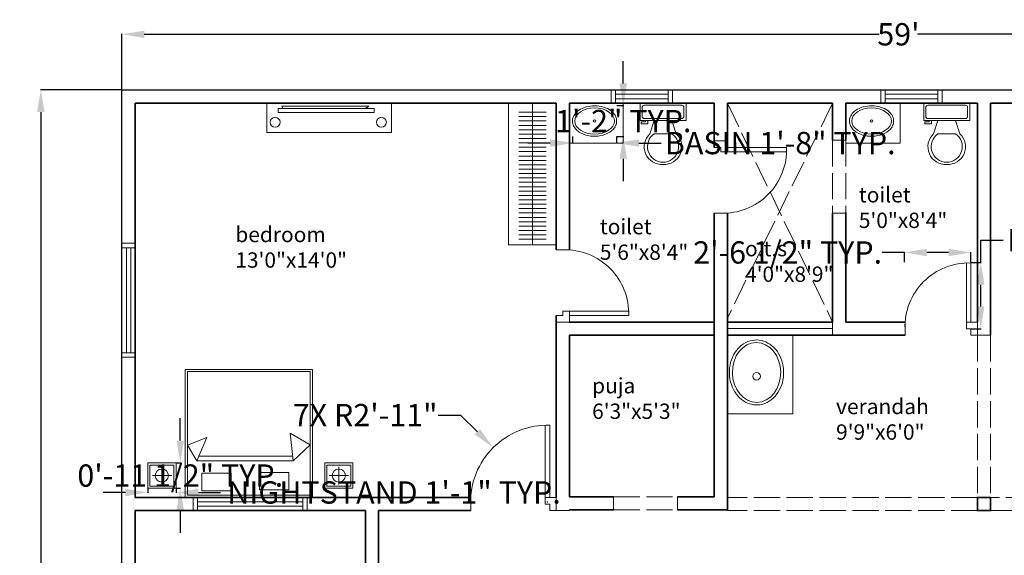
# Model space of a CAD drawing. Units: inches. Extents: x 29 to 4581, y 6 to 2196.
# Tile 2 of 3: x 3825 to 4274, y 1948 to 2192. Entities that reach past the tile are written whole.
import ezdxf

# ---------------------------------------------------------------- set-up
doc = ezdxf.new("R2010")
doc.units = ezdxf.units.IN
doc.header["$MEASUREMENT"] = 0
doc.linetypes.add('ACAD_ISO02W100', pattern=[15, 12, -3])
for name, color, linetype, lineweight in [('A-ANNO-DIMS', 2, 'Continuous', 18), ('A-DOOR', 3, 'Continuous', 18), ('A-EQPM', 9, 'Continuous', 18), ('A-FLOR-CASE', 8, 'Continuous', 18), ('A-FLOR-CASE-PATT', 8, 'Continuous', 13), ('A-FLOR-FIXT', 9, 'Continuous', 18), ('A-FLOR-OPEN', 8, 'ACAD_ISO02W100', 13), ('A-GLAZ', 4, 'Continuous', 18), ('A-WALL', 7, 'Continuous', 35), ('A-WALL-OVHD', 8, 'ACAD_ISO02W100', 18), ('C-PROP', 8, 'Continuous', 25)]:
    doc.layers.add(name, color=color, linetype=linetype, lineweight=lineweight)
for name, color, linetype, lineweight, true_color in [('A-AREA-IDEN', 41, 'Continuous', 18, 0xf4ee51), ('A-COLS', 240, 'Continuous', 35, 0xed1f24), ('A-FURN', 31, 'Continuous', 18, 0xfecc66)]:
    doc.layers.add(name, color=color, linetype=linetype, lineweight=lineweight, true_color=true_color)
doc.styles.get("Standard").update_dxf_attribs({"font": 'arial.ttf'})
doc.dimstyles.get("Standard").update_dxf_attribs({"dimtxt": 10.18, "dimasz": 10.18, "dimexe": 0.18, "dimexo": 0.0625, "dimgap": 0.09, "dimtad": 0, "dimtih": 1, "dimtoh": 1, "dimdec": 0, "dimzin": 0, "dimdsep": 46, "dimlunit": 3, "dimtxsty": 'Standard', "dimcen": 0.09, "dimadec": 0, "dimazin": 0, "dimtfac": 1, "dimtdec": 0, "dimtofl": 0, "dimtmove": 0, "dimatfit": 3, "dimfxl": 1, "dimtolj": 1, "dimtzin": 0, "dimarcsym": 0})

# ---------------------------------------------------------------- blocks, each defined once
blk = doc.blocks.new('*U2')
for p, q in [((9.5, -6), (9.5, -2)), ((-10, -8.5), (-8, -8.5)), ((-10, -9.5), (-10, -8.5)), ((-8, -8.5), (-8, -8)), ((-7, -8), (-7, -9.5)), ((-4, -8), (-6, -14)), ((4, -8), (6, -14)), ((-7, -9.5), (-10, -9.5)), ((4, -14), (-4, -14))]:
    blk.add_line(p, q)
blk.add_lwpolyline([(10.5, -8), (10.5, 0), (-10.5, 0), (-10.5, -8)], close=True)
for points in [[(-9.5, -2), (-9.5, -6)], [(8.5, -1), (-8.5, -1)], [(-8.5, -7), (8.5, -7)]]:
    blk.add_lwpolyline(points)
for centre, radius, start, end in [((-8.625, -1.875), 0.8839, 81.8699, 188.1301), ((8.625, -1.875), 0.8839, 351.8699, 98.1301), ((-8.625, -6.125), 0.8839, 171.869898, 278.1301), ((8.625, -6.125), 0.8839, 261.8699, 8.1301), ((-0.4772, -19.9188), 8.0953, 133.01722, 273.38), ((0.0374, -19.8731), 7.127, 124.50543, 269.7), ((-0.0373, -19.8731), 7.127, 270.3, 55.4946), ((0.4773, -19.9188), 8.0953, 266.62, 46.9828)]:
    blk.add_arc(centre, radius, start, end)
blk = doc.blocks.new('*D7')
at = {"layer": 'A-ANNO-DIMS', "color": 0, "lineweight": -2, "transparency": 16777216}
for p, q in [((3871.98, 2160.26), (3871.98, 2185.77)), ((3882.16, 2185.59), (4217.25, 2185.59)), ((4569.8, 2185.59), (4234.7, 2185.59)), ((4579.98, 2160.26), (4579.98, 2185.77))]:
    blk.add_line(p, q, dxfattribs=at)
at = {"layer": 'A-ANNO-DIMS', "color": 0, "transparency": 16777216}
for points in [[(3882.16, 2187.28), (3882.16, 2183.89), (3871.98, 2185.59)], [(4569.8, 2187.28), (4569.8, 2183.89), (4579.98, 2185.59)]]:
    blk.add_solid(points, dxfattribs=at)
at = {"layer": 'Defpoints', "color": 0, "transparency": 16777216}
for p in [(4579.98, 2185.59), (3871.98, 2160.2), (4579.98, 2160.2)]:
    blk.add_point(p, dxfattribs=at)
at = {"layer": 'A-ANNO-DIMS', "color": 0, "transparency": 16777216, "insert": (4225.98, 2185.59), "char_height": 10.18, "attachment_point": 5}
blk.add_mtext("\\A1;59'", dxfattribs=at)
blk = doc.blocks.new('*D8')
at = {"layer": 'A-ANNO-DIMS', "color": 0, "lineweight": -2, "transparency": 16777216}
for p, q in [((3871.91, 2160.26), (3834.8, 2160.26)), ((3834.98, 2150.08), (3834.98, 1865.52)), ((3834.98, 1570.38), (3834.98, 1854.94)), ((3871.91, 1560.2), (3834.8, 1560.2))]:
    blk.add_line(p, q, dxfattribs=at)
at = {"layer": 'A-ANNO-DIMS', "color": 0, "transparency": 16777216}
for points in [[(3833.29, 2150.08), (3836.68, 2150.08), (3834.98, 2160.26)], [(3833.29, 1570.38), (3836.68, 1570.38), (3834.98, 1560.2)]]:
    blk.add_solid(points, dxfattribs=at)
at = {"layer": 'Defpoints', "color": 0, "transparency": 16777216}
for p in [(3834.98, 2160.26), (3871.98, 2160.26), (3871.98, 1560.2)]:
    blk.add_point(p, dxfattribs=at)
at = {"layer": 'A-ANNO-DIMS', "color": 0, "transparency": 16777216, "insert": (3834.98, 1860.23), "char_height": 10.18, "attachment_point": 5}
blk.add_mtext("\\A1;50'", dxfattribs=at)
blk = doc.blocks.new('DOOR-36IN')
for p, q in [((34.01, 0), (34.01, 36)), ((36.01, 3), (36.01, 36)), ((34.01, 0), (36.01, 0))]:
    blk.add_line(p, q)
blk.add_arc((35.01, 1), 35.01, 88.3634, 181.6366)
blk = doc.blocks.new('DOOR-30IN')
for p, q in [((0, 2), (30, 2)), ((0, 2), (0, 0)), ((3, 0), (30, 0))]:
    blk.add_line(p, q)
blk.add_arc((1, 1), 29.02, 358.0251, 91.9749)
blk = doc.blocks.new('WIN-48')
for p, q in [((0, 6), (0, 0)), ((2, 6), (2, 0)), ((50, 6), (50, 0)), ((52, 6), (52, 0)), ((2, 4), (50, 4)), ((2, 2), (50, 2))]:
    blk.add_line(p, q)
blk = doc.blocks.new('WIN-24')
for p, q in [((6, 28), (0, 28)), ((6, 26), (0, 26)), ((2, 26), (2, 2)), ((4, 26), (4, 2)), ((6, 2), (0, 2)), ((6, 0), (0, 0))]:
    blk.add_line(p, q)
blk = doc.blocks.new('BASIN-OVAL')
blk.add_circle((10.07, 6.96), 0.572)
blk.add_ellipse((10.07, 6.96), major_axis=(9.07, 0), ratio=0.657752)
blk.add_open_spline([(20.13, 6.96), (20.13, 7.48), (20.05, 7.99), (19.74, 8.98), (19.5, 9.46), (18.6, 10.81), (17.74, 11.59), (15.67, 12.84), (14.47, 13.31), (11.89, 13.88), (10.52, 13.98), (7.83, 13.82), (6.51, 13.55), (4.11, 12.67), (3.03, 12.06), (1.49, 10.71), (0.93, 10.02), (0.24, 8.64), (0.05, 7.96), (-0.03, 6.59), (0.07, 5.9), (0.54, 4.6), (0.91, 3.98), (1.85, 2.86), (2.43, 2.36), (4.23, 1.16), (5.63, 0.61), (8.62, -0.01), (10.22, -0.08), (13.3, 0.28), (14.78, 0.7), (17.33, 1.99), (18.39, 2.86), (19.54, 4.5), (19.85, 5.16), (20.09, 6.22), (20.13, 6.59), (20.13, 6.96)], degree=3, knots=[0, 0, 0, 0, 0.206246, 0.206246, 0.412492, 0.412492, 0.829146, 0.829146, 1.245799, 1.245799, 1.662453, 1.662453, 2.079106, 2.079106, 2.495759, 2.495759, 2.824502, 2.824502, 3.099346, 3.099346, 3.37419, 3.37419, 3.649034, 3.649034, 3.923877, 3.923877, 4.405635, 4.405635, 4.887392, 4.887392, 5.369149, 5.369149, 5.850906, 5.850906, 6.134068, 6.134068, 6.283185, 6.283185, 6.283185, 6.283185])
blk = doc.blocks.new('NIGHTSTAND-WIDE')
for p, q in [((6.43, 9.73), (6.43, 1.64)), ((2.09, 5.78), (10.92, 5.78))]:
    blk.add_line(p, q)
for points in [[(0, 11.56), (12.87, 11.56), (12.87, 0), (0, 0)], [(1, 10.56), (11.87, 10.56), (11.87, 1), (1, 1)]]:
    blk.add_lwpolyline(points, close=True)
blk.add_circle((6.43, 5.78), 2.99)
blk = doc.blocks.new('*D28')
at = {"layer": 'A-ANNO-DIMS', "color": 0, "lineweight": -2, "transparency": 16777216}
for p, q in [((4263.52, 2081.47), (4263.52, 2091.65)), ((4263.52, 2091.65), (4273.7, 2091.65)), ((4259.04, 2081.47), (4263.7, 2081.47)), ((4263.52, 2061.38), (4263.52, 2071.29)), ((4259.04, 2051.2), (4263.7, 2051.2))]:
    blk.add_line(p, q, dxfattribs=at)
at = {"layer": 'A-ANNO-DIMS', "color": 0, "transparency": 16777216}
for points in [[(4261.82, 2071.29), (4265.21, 2071.29), (4263.52, 2081.47)], [(4261.82, 2061.38), (4265.21, 2061.38), (4263.52, 2051.2)]]:
    blk.add_solid(points, dxfattribs=at)
at = {"layer": 'Defpoints', "color": 0, "transparency": 16777216}
for p in [(4258.98, 2081.47), (4263.52, 2081.47), (4258.98, 2051.2)]:
    blk.add_point(p, dxfattribs=at)
at = {"layer": 'A-ANNO-DIMS', "color": 0, "transparency": 16777216, "insert": (4339.73, 2091.65), "char_height": 10.18, "attachment_point": 5}
blk.add_mtext('\\A1;DOOR 2\'-6 1/2" TYP.', dxfattribs=at)
blk = doc.blocks.new('*D29')
at = {"layer": 'A-ANNO-DIMS', "color": 0, "lineweight": -2, "transparency": 16777216}
for p, q in [((4228.7, 2086.02), (4218.52, 2086.02)), ((4228.7, 2081.54), (4228.7, 2086.2)), ((4248.8, 2086.02), (4238.88, 2086.02)), ((4258.98, 2081.54), (4258.98, 2086.2))]:
    blk.add_line(p, q, dxfattribs=at)
at = {"layer": 'A-ANNO-DIMS', "color": 0, "transparency": 16777216}
for points in [[(4238.88, 2087.71), (4238.88, 2084.32), (4228.7, 2086.02)], [(4248.8, 2087.71), (4248.8, 2084.32), (4258.98, 2086.02)]]:
    blk.add_solid(points, dxfattribs=at)
at = {"layer": 'Defpoints', "color": 0, "transparency": 16777216}
for p in [(4228.7, 2086.02), (4228.7, 2081.47), (4258.98, 2081.47)]:
    blk.add_point(p, dxfattribs=at)
at = {"layer": 'A-ANNO-DIMS', "color": 0, "transparency": 16777216, "insert": (4175.46, 2086.02), "char_height": 10.18, "attachment_point": 5}
blk.add_mtext('\\A1;2\'-6 1/2" TYP.', dxfattribs=at)
blk = doc.blocks.new('*D34')
at = {"layer": 'A-ANNO-DIMS', "color": 0, "lineweight": -2, "transparency": 16777216}
for p, q in [((4077.33, 2138.9), (4077.33, 2135.76)), ((4097.5, 2138.9), (4097.5, 2135.76)), ((4067.15, 2135.94), (4056.97, 2135.94)), ((4107.68, 2135.94), (4117.86, 2135.94))]:
    blk.add_line(p, q, dxfattribs=at)
at = {"layer": 'A-ANNO-DIMS', "color": 0, "transparency": 16777216}
for points in [[(4067.15, 2137.64), (4067.15, 2134.24), (4077.33, 2135.94)], [(4107.68, 2137.64), (4107.68, 2134.24), (4097.5, 2135.94)]]:
    blk.add_solid(points, dxfattribs=at)
at = {"layer": 'Defpoints', "color": 0, "transparency": 16777216}
for p in [(4077.33, 2138.97), (4097.5, 2138.97), (4097.5, 2135.94)]:
    blk.add_point(p, dxfattribs=at)
at = {"layer": 'A-ANNO-DIMS', "color": 0, "transparency": 16777216, "insert": (4172.07, 2135.94), "char_height": 10.18, "attachment_point": 5}
blk.add_mtext('\\A1;BASIN 1\'-8" TYP.', dxfattribs=at)
blk = doc.blocks.new('*D35')
at = {"layer": 'A-ANNO-DIMS', "color": 0, "lineweight": -2, "transparency": 16777216}
for p, q in [((4100.53, 2163.21), (4100.53, 2173.39)), ((4097.56, 2153.03), (4100.71, 2153.03)), ((4097.56, 2138.97), (4100.71, 2138.97)), ((4100.53, 2128.79), (4100.53, 2118.61))]:
    blk.add_line(p, q, dxfattribs=at)
at = {"layer": 'A-ANNO-DIMS', "color": 0, "transparency": 16777216}
for points in [[(4098.83, 2163.21), (4102.22, 2163.21), (4100.53, 2153.03)], [(4098.83, 2128.79), (4102.22, 2128.79), (4100.53, 2138.97)]]:
    blk.add_solid(points, dxfattribs=at)
at = {"layer": 'Defpoints', "color": 0, "transparency": 16777216}
for p in [(4097.5, 2153.03), (4100.53, 2153.03), (4097.5, 2138.97)]:
    blk.add_point(p, dxfattribs=at)
at = {"layer": 'A-ANNO-DIMS', "color": 0, "transparency": 16777216, "insert": (4100.53, 2146), "char_height": 10.18, "attachment_point": 5}
blk.add_mtext('\\A1;1\'-2" TYP.', dxfattribs=at)
blk = doc.blocks.new('*D40')
at = {"layer": 'A-ANNO-DIMS', "color": 0, "lineweight": -2, "transparency": 16777216}
for p, q in [((3873.56, 1976.48), (3863.38, 1976.48)), ((3883.74, 1978.35), (3883.74, 1976.3)), ((3896.61, 1978.35), (3896.61, 1976.3)), ((3906.79, 1976.48), (3916.97, 1976.48))]:
    blk.add_line(p, q, dxfattribs=at)
at = {"layer": 'A-ANNO-DIMS', "color": 0, "transparency": 16777216}
for points in [[(3873.56, 1978.17), (3873.56, 1974.78), (3883.74, 1976.48)], [(3906.79, 1978.17), (3906.79, 1974.78), (3896.61, 1976.48)]]:
    blk.add_solid(points, dxfattribs=at)
at = {"layer": 'Defpoints', "color": 0, "transparency": 16777216}
for p in [(3883.74, 1978.41), (3896.61, 1978.41), (3896.61, 1976.48)]:
    blk.add_point(p, dxfattribs=at)
at = {"layer": 'A-ANNO-DIMS', "color": 0, "transparency": 16777216, "insert": (3996.03, 1976.48), "char_height": 10.18, "attachment_point": 5}
blk.add_mtext('\\A1;NIGHTSTAND 1\'-1" TYP.', dxfattribs=at)
blk = doc.blocks.new('*D41')
at = {"layer": 'A-ANNO-DIMS', "color": 0, "lineweight": -2, "transparency": 16777216}
for p, q in [((3898.54, 2000.15), (3898.54, 2010.33)), ((3896.67, 1989.97), (3898.72, 1989.97)), ((3896.67, 1978.41), (3898.72, 1978.41)), ((3898.54, 1968.23), (3898.54, 1958.05))]:
    blk.add_line(p, q, dxfattribs=at)
at = {"layer": 'A-ANNO-DIMS', "color": 0, "transparency": 16777216}
for points in [[(3896.84, 2000.15), (3900.23, 2000.15), (3898.54, 1989.97)], [(3896.84, 1968.23), (3900.23, 1968.23), (3898.54, 1978.41)]]:
    blk.add_solid(points, dxfattribs=at)
at = {"layer": 'Defpoints', "color": 0, "transparency": 16777216}
for p in [(3896.61, 1989.97), (3898.54, 1989.97), (3896.61, 1978.41)]:
    blk.add_point(p, dxfattribs=at)
at = {"layer": 'A-ANNO-DIMS', "color": 0, "transparency": 16777216, "insert": (3898.54, 1984.19), "char_height": 10.18, "attachment_point": 5}
blk.add_mtext('\\A1;0\'-11 1/2" TYP.', dxfattribs=at)
blk = doc.blocks.new('*D48')
at = {"layer": 'A-ANNO-DIMS', "color": 0, "lineweight": -2, "transparency": 16777216}
for p, q in [((4016.18, 2011.81), (4026.36, 2011.81)), ((4026.36, 2011.81), (4034.02, 2004.15)), ((4065.89, 1972.2), (4066.07, 1972.2)), ((4065.98, 1972.11), (4065.98, 1972.29))]:
    blk.add_line(p, q, dxfattribs=at)
at = {"layer": 'A-ANNO-DIMS', "color": 0, "transparency": 16777216}
blk.add_solid([(4035.22, 2005.35), (4032.82, 2002.95), (4041.22, 1996.96)], dxfattribs=at)
at = {"layer": 'Defpoints', "color": 0, "transparency": 16777216}
for p in [(4041.22, 1996.96), (4065.98, 1972.2)]:
    blk.add_point(p, dxfattribs=at)
at = {"layer": 'A-ANNO-DIMS', "color": 0, "transparency": 16777216, "insert": (3982.84, 2011.81), "char_height": 10.18, "attachment_point": 5}
blk.add_mtext('\\A1;7X R2\'-11"', dxfattribs=at)

msp = doc.modelspace()

# ---------------------------------------------------------------- hatches: boundary and pattern name
at = {"layer": 'A-FLOR-CASE-PATT'}
h = msp.add_hatch(dxfattribs=at)
h.set_pattern_fill('ANSI31', color=256, scale=16.0003, angle=-45, style=0)
h.paths.add_polyline_path([(4052.97, 2091.04), (4065.4, 2091.04), (4065.4, 2151.04), (4052.97, 2151.04)])

# ---------------------------------------------------------------- linework, layer by layer
at = {"layer": 'A-COLS'}
msp.add_lwpolyline([(4267.98, 1974.2), (4261.98, 1974.2), (4261.98, 1968.2), (4267.98, 1968.2)], close=True, dxfattribs=at)
at = {"layer": 'A-DOOR'}
for p, q in [((4147.98, 2136.93), (4141.98, 2136.93)), ((4144.98, 2133.93), (4141.98, 2133.93)), ((4147.98, 2103.93), (4141.98, 2103.93)), ((4075.98, 2087.2), (4069.98, 2087.2)), ((4072.98, 2057.2), (4069.98, 2057.2)), ((4075.98, 2059.2), (4075.98, 2054.2)), ((4075.98, 2054.2), (4069.98, 2054.2)), ((4228.98, 2054.2), (4228.98, 2048.2)), ((4256.98, 2054.2), (4261.98, 2054.2)), ((4261.98, 2054.2), (4261.98, 2048.2)), ((4258.98, 2051.2), (4258.98, 2048.2)), ((4258.98, 2048.2), (4261.98, 2048.2)), ((4030.98, 1974.2), (4030.98, 1968.2)), ((4064.98, 1974.2), (4069.98, 1974.2)), ((4066.98, 1971.2), (4066.98, 1968.2)), ((4069.98, 1974.2), (4069.98, 1968.2)), ((4066.98, 1968.2), (4075.98, 1968.2))]:
    msp.add_line(p, q, dxfattribs=at)
at = {"layer": 'A-EQPM'}
for p, q in [((3945.29, 2151.69), (3944.84, 2152.73)), ((3944.84, 2152.73), (3984.49, 2152.73)), ((3984.49, 2152.73), (3982.98, 2151.69))]:
    msp.add_line(p, q, dxfattribs=at)
for points in [[(3938.02, 2154.2), (3994.84, 2154.2), (3994.84, 2140.8), (3938.02, 2140.8)], [(3943.21, 2151.69), (3987.01, 2151.69), (3987.01, 2149.92), (3943.21, 2149.92)]]:
    msp.add_lwpolyline(points, close=True, dxfattribs=at)
for centre in [(3941.79, 2145.45), (3990.24, 2145.45)]:
    msp.add_circle(centre, 2.26, dxfattribs=at)
at = {"layer": 'A-FLOR-CASE'}
msp.add_line((4059.09, 2154.2), (4059.09, 2089.54), dxfattribs=at)
msp.add_lwpolyline([(4069.98, 2154.2), (4048.2, 2154.2), (4048.2, 2089.54), (4069.98, 2089.54)], close=True, dxfattribs=at)
at = {"layer": 'A-FLOR-FIXT'}
for p, q in [((4100.43, 2154.2), (4100.43, 2135.9)), ((4226.71, 2154.2), (4226.71, 2135.9)), ((4100.43, 2135.9), (4075.98, 2135.9)), ((4226.71, 2135.9), (4202.26, 2135.9)), ((4177.83, 2048.2), (4177.83, 2012.33)), ((4177.83, 2012.33), (4147.98, 2012.33))]:
    msp.add_line(p, q, dxfattribs=at)
msp.add_circle((4161.28, 2029.53), 1.74, dxfattribs=at)
msp.add_ellipse((4161.28, 2031.27), major_axis=(-0.18, 13.67), ratio=0.805439, start_param=-3.141592653589793, end_param=3.141592653589793, dxfattribs=at)
msp.add_open_spline([(4161.48, 2016.44), (4162.36, 2016.45), (4163.24, 2016.58), (4165.45, 2017.19), (4166.76, 2017.84), (4169.12, 2019.63), (4170.18, 2020.77), (4171.92, 2023.43), (4172.6, 2024.94), (4173.49, 2028.17), (4173.7, 2029.88), (4173.55, 2033.27), (4173.34, 2034.97), (4172.31, 2038.15), (4171.57, 2039.63), (4169.72, 2042.19), (4168.62, 2043.28), (4166.18, 2044.95), (4164.85, 2045.54), (4162.12, 2046.14), (4160.71, 2046.17), (4157.97, 2045.66), (4156.63, 2045.13), (4154.17, 2043.55), (4153.05, 2042.51), (4151.16, 2040.01), (4150.39, 2038.56), (4149.3, 2035.43), (4148.98, 2033.75), (4148.85, 2030.35), (4149.03, 2028.63), (4149.86, 2025.37), (4150.51, 2023.83), (4152.2, 2021.11), (4153.24, 2019.92), (4155.57, 2018.04), (4156.87, 2017.35), (4159.28, 2016.59), (4160.38, 2016.43), (4161.48, 2016.44)], degree=3, knots=[-3.141593, -3.141593, -3.141593, -3.141593, -2.924616, -2.924616, -2.58365, -2.58365, -2.242684, -2.242684, -1.901718, -1.901718, -1.560752, -1.560752, -1.219786, -1.219786, -0.87882, -0.87882, -0.537854, -0.537854, -0.196888, -0.196888, 0.144078, 0.144078, 0.485044, 0.485044, 0.82601, 0.82601, 1.166976, 1.166976, 1.507942, 1.507942, 1.848908, 1.848908, 2.189874, 2.189874, 2.53084, 2.53084, 2.871806, 2.871806, 3.141593, 3.141593, 3.141593, 3.141593], dxfattribs=at)
at = {"layer": 'A-FLOR-OPEN'}
for p, q in [((4147.98, 2154.2), (4195.98, 2054.2)), ((4195.98, 2154.2), (4147.98, 2055.97))]:
    msp.add_line(p, q, dxfattribs=at)
at = {"layer": 'A-FURN'}
for p, q in [((3957.83, 1998.26), (3948.64, 2003.56)), ((3948.64, 2003.56), (3950.05, 1990.93)), ((3901.82, 1998.09), (3910.72, 2001.64)), ((3906.13, 1990.93), (3901.82, 1998.09)), ((3910.72, 2001.64), (3906.13, 1990.93)), ((3950.05, 1990.93), (3957.83, 1998.26)), ((3906.13, 1990.93), (3950.05, 1990.93)), ((3907.05, 1993.06), (3949.82, 1993.01))]:
    msp.add_line(p, q, dxfattribs=at)
for points in [[(3900.82, 1974.2), (3958.83, 1974.2), (3958.83, 2032.66), (3900.82, 2032.66)], [(3901.82, 1975.2), (3957.83, 1975.2), (3957.83, 2031.66), (3901.82, 2031.66)], [(3908.34, 1985.25), (3921.69, 1985.25), (3921.69, 1977.3), (3908.34, 1977.3)], [(3934.62, 1985.67), (3947.98, 1985.67), (3947.98, 1977.73), (3934.62, 1977.73)]]:
    msp.add_lwpolyline(points, close=True, dxfattribs=at)
at = {"layer": 'A-GLAZ'}
for p, q in [((4195.98, 2054.2), (4195.98, 2048.2)), ((4147.98, 2051.26), (4195.98, 2051.26))]:
    msp.add_line(p, q, dxfattribs=at)
at = {"layer": 'A-WALL'}
for p, q in [((3877.98, 2154.2), (4069.98, 2154.2)), ((3877.98, 1974.2), (3877.98, 2154.2)), ((4069.98, 2154.2), (4069.98, 2087.2)), ((4075.98, 2154.2), (4075.98, 2087.14)), ((4075.98, 2154.2), (4141.98, 2154.2)), ((4141.98, 2154.2), (4141.98, 2133.93)), ((4147.98, 2154.2), (4147.98, 2131.93)), ((4147.98, 2154.2), (4195.98, 2154.2)), ((4195.98, 2154.2), (4195.98, 2137.28)), ((4201.98, 2154.2), (4201.98, 2137.28)), ((4201.98, 2154.2), (4261.98, 2154.2)), ((4261.98, 2154.2), (4261.98, 2054.2)), ((4267.98, 2154.2), (4267.98, 2048.2)), ((4267.98, 2154.2), (4423.98, 2154.2)), ((4141.98, 2103.93), (4141.98, 2048.2)), ((4147.98, 2103.98), (4147.98, 2048.2)), ((4195.98, 2103.93), (4195.98, 2054.2)), ((4201.98, 2104.2), (4201.98, 2054.2)), ((4069.98, 2057.2), (4069.98, 1974.2)), ((4075.98, 2054.2), (4141.98, 2054.2)), ((4147.98, 2054.2), (4195.98, 2054.2)), ((4201.98, 2054.2), (4229.03, 2054.2)), ((4075.98, 2048.2), (4141.98, 2048.2)), ((4075.98, 2048.2), (4075.98, 1974.52)), ((4141.98, 2048.2), (4141.98, 1974.52)), ((4147.98, 2048.2), (4147.98, 1968.52)), ((4147.98, 2048.2), (4228.98, 2048.2)), ((3877.98, 1974.2), (4031.02, 1974.2)), ((4075.98, 1974.52), (4096.04, 1974.52)), ((4125.3, 1974.52), (4141.98, 1974.52)), ((4261.98, 1974.2), (4261.98, 1968.2)), ((3877.98, 1968.2), (3982.98, 1968.2)), ((3877.98, 1833.2), (3877.98, 1968.2)), ((3982.98, 1931.7), (3982.98, 1968.2)), ((3988.98, 1968.2), (4030.98, 1968.2)), ((3988.98, 1933.7), (3988.98, 1968.2)), ((4075.98, 1968.52), (4096.04, 1968.52)), ((4075.98, 1968.52), (4075.98, 1968.2)), ((4125.3, 1968.52), (4147.98, 1968.52)), ((4261.98, 1968.2), (4267.98, 1968.2))]:
    msp.add_line(p, q, dxfattribs=at)
at = {"layer": 'A-WALL-OVHD'}
for p, q in [((4195.98, 2137.28), (4201.98, 2137.28)), ((4195.98, 2137.28), (4195.98, 2103.93)), ((4201.98, 2137.28), (4201.98, 2104.2)), ((4195.98, 2103.93), (4201.98, 2103.93)), ((4261.98, 2048.2), (4267.98, 2048.2)), ((4261.98, 2048.2), (4261.98, 1974.2)), ((4267.98, 2048.2), (4267.98, 1974.2)), ((4096.04, 1974.52), (4096.04, 1968.52)), ((4096.04, 1974.52), (4125.3, 1974.52)), ((4125.3, 1974.52), (4125.3, 1968.52)), ((4261.98, 1974.2), (4147.98, 1974.2)), ((4302.01, 1974.2), (4267.98, 1974.2)), ((4096.04, 1968.52), (4125.3, 1968.52)), ((4261.98, 1968.2), (4147.98, 1968.2)), ((4267.98, 1968.2), (4302.01, 1968.2))]:
    msp.add_line(p, q, dxfattribs=at)
at = {"layer": 'C-PROP'}
for p, q in [((3871.98, 1560.2), (3871.98, 2160.2)), ((3871.98, 2160.2), (4579.98, 2160.2))]:
    msp.add_line(p, q, dxfattribs=at)

# ---------------------------------------------------------------- block references
at = {"layer": 'A-DOOR', "extrusion": (0, 0, -1), "zscale": -1, "rotation": 180}
msp.add_blockref('DOOR-30IN', (-4144.98, 2133.93), dxfattribs=at)
at = {"layer": 'A-DOOR'}
for name, p in [('DOOR-30IN', (4072.98, 2057.2)), ('DOOR-36IN', (4030.96, 1971.2))]:
    msp.add_blockref(name, p, dxfattribs=at)
at = {"layer": 'A-DOOR', "rotation": 89.99999999999432}
msp.add_blockref('DOOR-30IN', (4258.98, 2051.2), dxfattribs=at)
at = {"layer": 'A-FLOR-FIXT'}
for name, p in [('BASIN-OVAL', (4077.37, 2139.05)), ('*U2', (4118.65, 2154.2)), ('BASIN-OVAL', (4203.65, 2139.05)), ('*U2', (4247.99, 2154.2))]:
    msp.add_blockref(name, p, dxfattribs=at)
at = {"layer": 'A-FURN'}
for p in [(3883.74, 1978.41), (3964.4, 1978.41)]:
    msp.add_blockref('NIGHTSTAND-WIDE', p, dxfattribs=at)
at = {"layer": 'A-GLAZ'}
for name, p, rotation in [('WIN-24', (4094.98, 2160.2), 270.0000000000017), ('WIN-24', (4245.98, 2154.2), 89.99999999999898), ('WIN-48', (3877.98, 2038.2), 90.00000000000011)]:
    msp.add_blockref(name, p, dxfattribs=dict(at, rotation=rotation))
msp.add_blockref('WIN-48', (3904.48, 1968.2), dxfattribs=at)

# ---------------------------------------------------------------- texts
at = {"layer": 'A-AREA-IDEN', "char_height": 7, "attachment_point": 1}
for s, insert in [('toilet\\P5\'0"x8\'4"', (4207.91, 2115.85)), ('toilet\\P5\'6"x8\'4"', (4089.83, 2101.32)), ('bedroom\\P13\'0"x14\'0"', (3923.65, 2097.73)), ('o.t.s\\P4\'0"x8\'9"', (4156.03, 2091.28)), ('puja\\P6\'3"x5\'3"', (4086.31, 2028.72)), ('verandah\\P9\'9"x6\'0"', (4197.54, 2019.23))]:
    msp.add_mtext_dynamic_manual_height_columns(s, width=59.5635, gutter_width=1, heights=[0], dxfattribs=dict(at, insert=insert))

# ---------------------------------------------------------------- dimensions: what is measured, and where the dimension line sits
at = {"layer": 'A-ANNO-DIMS'}
dim = msp.add_linear_dim(base=(4579.98, 2185.59), p1=(3871.98, 2160.2), p2=(4579.98, 2160.2), dimstyle='Standard', override={"dimclrd": 0, "dimclre": 0, "dimclrt": 0}, dxfattribs=at)
dim.commit()
dim.dimension.update_dxf_attribs({"geometry": '*D7', "text_midpoint": (4225.98, 2185.59)})
for base, p1, p2, angle, text, picture, middle in [((4100.53, 2153.03), (4097.5, 2138.97), (4097.5, 2153.03), 90, '<> TYP.', '*D35', (4100.53, 2146)), ((4263.52, 2081.47), (4258.98, 2051.2), (4258.98, 2081.47), 90, 'DOOR <> TYP.', '*D28', (4339.73, 2091.65)), ((4228.7, 2086.02), (4258.98, 2081.47), (4228.7, 2081.47), 180, '<> TYP.', '*D29', (4175.46, 2086.02)), ((3898.54, 1989.97), (3896.61, 1978.41), (3896.61, 1989.97), 90, '<> TYP.', '*D41', (3898.54, 1984.19))]:
    dim = msp.add_linear_dim(base=base, p1=p1, p2=p2, angle=angle, text=text, dimstyle='Standard', override={"dimdec": 1, "dimlfac": 1, "dimrnd": 0, "dimzin": 1, "dimdsep": 46, "dimlunit": 4, "dimfrac": 2}, dxfattribs=at)
    dim.commit()
    dim.dimension.update_dxf_attribs({"geometry": picture, "text_midpoint": middle})
dim = msp.add_linear_dim(base=(3834.98, 2160.26), p1=(3871.98, 1560.2), p2=(3871.98, 2160.26), angle=90, dimstyle='Standard', override={"dimclrd": 0, "dimclre": 0, "dimclrt": 0}, dxfattribs=at)
dim.commit()
dim.dimension.update_dxf_attribs({"geometry": '*D8', "text_midpoint": (3834.98, 1860.23)})
for base, p1, p2, text, picture, middle in [((4097.5, 2135.94), (4077.33, 2138.97), (4097.5, 2138.97), 'BASIN <> TYP.', '*D34', (4172.07, 2135.94)), ((3896.61, 1976.48), (3883.74, 1978.41), (3896.61, 1978.41), 'NIGHTSTAND <> TYP.', '*D40', (3996.03, 1976.48))]:
    dim = msp.add_linear_dim(base=base, p1=p1, p2=p2, text=text, dimstyle='Standard', override={"dimdec": 1, "dimlfac": 1, "dimrnd": 0, "dimzin": 1, "dimdsep": 46, "dimlunit": 4, "dimfrac": 2}, dxfattribs=at)
    dim.commit()
    dim.dimension.update_dxf_attribs({"geometry": picture, "text_midpoint": middle})
dim = msp.add_radius_dim(center=(4065.98, 1972.2), mpoint=(4041.22, 1996.96), text='7X <>', dimstyle='Standard', override={"dimdec": 1, "dimlfac": 1, "dimrnd": 0, "dimzin": 1, "dimdsep": 46, "dimlunit": 4, "dimfrac": 2}, dxfattribs=at)
dim.commit()
dim.dimension.update_dxf_attribs({"geometry": '*D48', "text_midpoint": (3982.84, 2011.81), "dimtype": 164})

doc.saveas('drawing.dxf')
